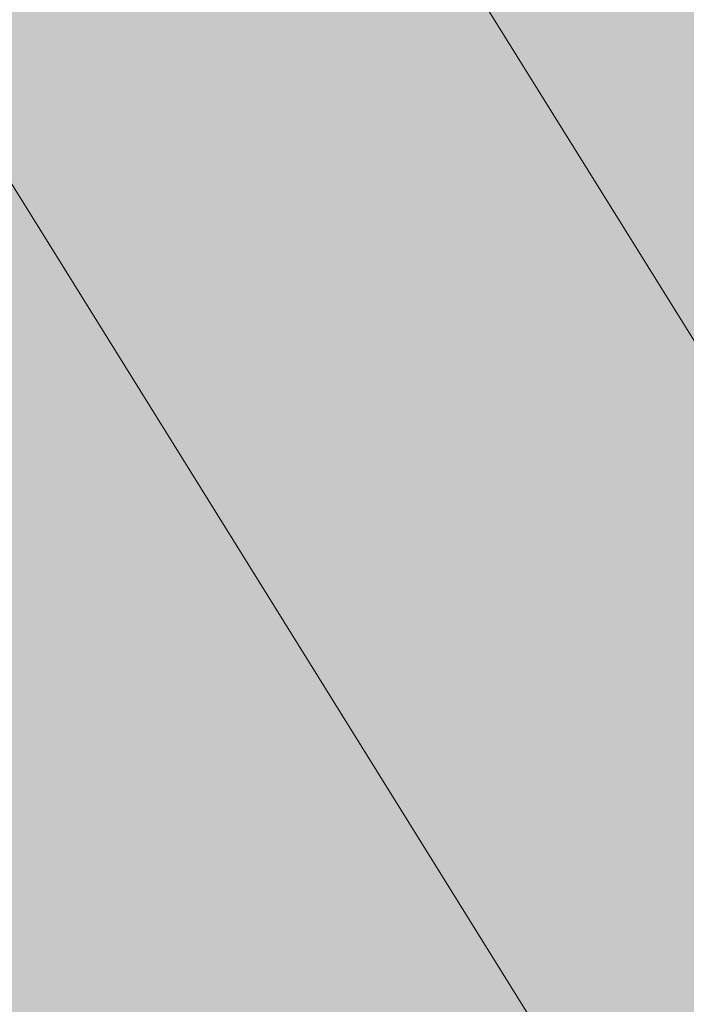
# Model space of a CAD drawing. Units: millimetres. Extents: x 11032 to 26788, y 3406 to 24505.
# Tile 49 of 78: x 15719 to 15786, y 16177 to 16276. Entities that reach past the tile are written whole.
import ezdxf

# ---------------------------------------------------------------- set-up
doc = ezdxf.new("R2010")
doc.units = ezdxf.units.MM
doc.header["$MEASUREMENT"] = 0
for name, color, linetype, lineweight in [('A-ANNO-DIMS', 2, 'Continuous', 18), ('A-GLAZ', 250, 'Continuous', 20), ('A-ROOF', 7, 'Continuous', 30), ('A-WALL', 7, 'Continuous', 35), ('E-LITE', 7, 'Continuous', 18), ('E-LITE-PATT', 7, 'Continuous', 13)]:
    doc.layers.add(name, color=color, linetype=linetype, lineweight=lineweight)
doc.layers.add('A-GLAZ-FRAM-PATT', color=250, linetype='Continuous', lineweight=13, true_color=0x262627)
doc.layers.add('A-ROOF-PATT', color=9, linetype='Continuous', lineweight=13, true_color=0xc7c8ca)
doc.styles.get("Standard").update_dxf_attribs({"font": 'arial.ttf'})
doc.dimstyles.get("Standard").update_dxf_attribs({"dimtxt": 150, "dimasz": 100, "dimexe": 10, "dimexo": 5, "dimgap": 5, "dimtad": 0, "dimtih": 1, "dimtoh": 1, "dimdec": 0, "dimzin": 0, "dimdsep": 46, "dimtxsty": 'Standard', "dimcen": 0.09, "dimadec": 0, "dimazin": 0, "dimtfac": 1, "dimtdec": 0, "dimtofl": 0, "dimtmove": 0, "dimatfit": 3, "dimfxl": 1, "dimtolj": 1, "dimtzin": 0, "dimarcsym": 0})

# ---------------------------------------------------------------- blocks, each defined once
blk = doc.blocks.new('*D36')
at = {"layer": 'A-ANNO-DIMS', "color": 0, "lineweight": -2, "transparency": 16777216}
for p, q in [((12301.265, 17115.885), (12301.265, 24416.858)), ((25397.404, 4466.399), (25397.404, 24416.858)), ((12401.265, 24406.858), (18569.198, 24406.858)), ((25297.404, 24406.858), (19129.471, 24406.858))]:
    blk.add_line(p, q, dxfattribs=at)
at = {"layer": 'A-ANNO-DIMS', "color": 0, "transparency": 16777216}
for points in [[(12401.265, 24423.525), (12401.265, 24390.191), (12301.265, 24406.858)], [(25297.404, 24423.525), (25297.404, 24390.191), (25397.404, 24406.858)]]:
    blk.add_solid(points, dxfattribs=at)
at = {"layer": 'Defpoints', "color": 0, "transparency": 16777216}
for p in [(25397.404, 24406.858), (12301.265, 17110.885), (25397.404, 4461.399)]:
    blk.add_point(p, dxfattribs=at)
at = {"layer": 'A-ANNO-DIMS', "color": 0, "transparency": 16777216, "insert": (18849.334, 24406.858), "char_height": 150, "attachment_point": 5}
blk.add_mtext('\\A1;13096', dxfattribs=at)
blk = doc.blocks.new('*D37')
at = {"layer": 'A-ANNO-DIMS', "color": 0, "lineweight": -2, "transparency": 16777216}
for p, q in [((18087.739, 23450.358), (11334.765, 23450.358)), ((11344.765, 23350.358), (11344.765, 14037.465)), ((11344.765, 4561.399), (11344.765, 13874.293)), ((12927.665, 4461.399), (11334.765, 4461.399))]:
    blk.add_line(p, q, dxfattribs=at)
at = {"layer": 'A-ANNO-DIMS', "color": 0, "transparency": 16777216}
for points in [[(11328.098, 23350.358), (11361.431, 23350.358), (11344.765, 23450.358)], [(11328.098, 4561.399), (11361.431, 4561.399), (11344.765, 4461.399)]]:
    blk.add_solid(points, dxfattribs=at)
at = {"layer": 'Defpoints', "color": 0, "transparency": 16777216}
for p in [(11344.765, 23450.358), (18092.739, 23450.358), (12932.665, 4461.399)]:
    blk.add_point(p, dxfattribs=at)
at = {"layer": 'A-ANNO-DIMS', "color": 0, "transparency": 16777216, "insert": (11344.765, 13955.879), "char_height": 150, "attachment_point": 5}
blk.add_mtext('\\A1;18989', dxfattribs=at)
blk = doc.blocks.new('*D45')
at = {"layer": 'A-ANNO-DIMS', "color": 0, "lineweight": -2, "transparency": 16777216}
for p, q in [((13792.367, 18518.925), (26363.904, 18518.925)), ((26353.904, 18418.925), (26353.904, 17450.319)), ((26353.904, 16318.44), (26353.904, 17287.045)), ((22902.404, 16218.44), (26363.904, 16218.44))]:
    blk.add_line(p, q, dxfattribs=at)
at = {"layer": 'A-ANNO-DIMS', "color": 0, "transparency": 16777216}
for points in [[(26337.237, 18418.925), (26370.57, 18418.925), (26353.904, 18518.925)], [(26337.237, 16318.44), (26370.57, 16318.44), (26353.904, 16218.44)]]:
    blk.add_solid(points, dxfattribs=at)
at = {"layer": 'Defpoints', "color": 0, "transparency": 16777216}
for p in [(13787.367, 18518.925), (26353.904, 18518.925), (22897.404, 16218.44)]:
    blk.add_point(p, dxfattribs=at)
at = {"layer": 'A-ANNO-DIMS', "color": 0, "transparency": 16777216, "insert": (26353.904, 17368.682), "char_height": 150, "attachment_point": 5}
blk.add_mtext('\\A1;2300.5', dxfattribs=at)
blk = doc.blocks.new('*D57')
at = {"layer": 'A-ANNO-DIMS', "color": 0, "lineweight": -2, "transparency": 16777216}
for p, q in [((14994.704, 7266.399), (14994.704, 24416.858)), ((20894.704, 7266.399), (20894.704, 24416.858)), ((15094.704, 24406.858), (17715.983, 24406.858)), ((20794.704, 24406.858), (18173.425, 24406.858))]:
    blk.add_line(p, q, dxfattribs=at)
at = {"layer": 'A-ANNO-DIMS', "color": 0, "transparency": 16777216}
for points in [[(15094.704, 24423.525), (15094.704, 24390.191), (14994.704, 24406.858)], [(20794.704, 24423.525), (20794.704, 24390.191), (20894.704, 24406.858)]]:
    blk.add_solid(points, dxfattribs=at)
at = {"layer": 'Defpoints', "color": 0, "transparency": 16777216}
for p in [(20894.704, 24406.858), (14994.704, 7261.399), (20894.704, 7261.399)]:
    blk.add_point(p, dxfattribs=at)
at = {"layer": 'A-ANNO-DIMS', "color": 0, "transparency": 16777216, "insert": (17944.704, 24406.858), "char_height": 150, "attachment_point": 5}
blk.add_mtext('\\A1;5900', dxfattribs=at)
blk = doc.blocks.new('*D60')
at = {"layer": 'A-ANNO-DIMS', "color": 0, "lineweight": -2, "transparency": 16777216}
for p, q in [((14994.704, 7266.399), (14994.704, 24416.858)), ((16344.704, 7266.399), (16344.704, 24416.858)), ((15094.704, 24406.858), (15448.043, 24406.858)), ((16244.704, 24406.858), (15891.365, 24406.858))]:
    blk.add_line(p, q, dxfattribs=at)
at = {"layer": 'A-ANNO-DIMS', "color": 0, "transparency": 16777216}
for points in [[(15094.704, 24423.525), (15094.704, 24390.191), (14994.704, 24406.858)], [(16244.704, 24423.525), (16244.704, 24390.191), (16344.704, 24406.858)]]:
    blk.add_solid(points, dxfattribs=at)
at = {"layer": 'Defpoints', "color": 0, "transparency": 16777216}
for p in [(16344.704, 24406.858), (14994.704, 7261.399), (16344.704, 7261.399)]:
    blk.add_point(p, dxfattribs=at)
at = {"layer": 'A-ANNO-DIMS', "color": 0, "transparency": 16777216, "insert": (15669.704, 24406.858), "char_height": 150, "attachment_point": 5}
blk.add_mtext('\\A1;1350', dxfattribs=at)

msp = doc.modelspace()

# ---------------------------------------------------------------- hatches: boundary and pattern name
at = {"layer": 'A-GLAZ-FRAM-PATT'}
h = msp.add_hatch(color=256, dxfattribs=at)
edge = h.paths.add_edge_path()
edge.add_line((15284.393, 17051.32), (15084.393, 17001.32))
edge.add_line((15084.393, 17001.32), (15084.393, 15951.32))
edge.add_spline(control_points=[(15084.393, 15951.32), (15157.266, 15924.219), (15224.458, 15897.808), (15284.393, 15870.289)], knot_values=[511.94901, 511.94901, 511.94901, 511.94901, 697.371598, 697.371598, 697.371598, 697.371598], degree=3, periodic=0)
edge.add_line((15284.393, 15870.289), (15284.393, 17051.32))
edge = h.paths.add_edge_path()
edge.add_line((15659.393, 16354.387), (15459.393, 16675.629))
edge.add_line((15459.393, 16675.629), (15459.393, 15771.505))
edge.add_spline(control_points=[(15459.393, 15771.505), (15501.891, 15741.568), (15571.096, 15682.692), (15632.72, 15612.509), (15659.393, 15578.299)], knot_values=[905.064582, 905.064582, 905.064582, 905.064582, 1079.468271, 1223.158435, 1223.158435, 1223.158435, 1223.158435], degree=3, periodic=0)
edge.add_line((15659.393, 15578.299), (15659.393, 16354.387))
h.paths.add_polyline_path([(15284.393, 17051.32), (15284.393, 16956.717), (15784.393, 16153.61), (15784.393, 16248.213)])
h = msp.add_hatch(color=256, dxfattribs=at)
edge = h.paths.add_edge_path()
edge.add_spline(control_points=[(15409.393, 16728.446), (15384.197, 16718.122), (15359.177, 16707.259), (15334.393, 16695.842)], knot_values=[2052.671403, 2052.671403, 2052.671403, 2052.671403, 2131.020164, 2131.020164, 2131.020164, 2131.020164], degree=3, periodic=0)
edge.add_line((15334.393, 16695.842), (15334.393, 15846.165))
edge.add_spline(control_points=[(15334.393, 15846.165), (15360.99, 15832.635), (15385.89, 15818.741), (15409.393, 15804.345)], knot_values=[750.83835, 750.83835, 750.83835, 750.83835, 839.475874, 839.475874, 839.475874, 839.475874], degree=3, periodic=0)
edge.add_line((15409.393, 15804.345), (15409.393, 16728.446))
edge = h.paths.add_edge_path()
edge.add_line((15784.393, 16153.61), (15709.393, 16274.076))
edge.add_line((15709.393, 16274.076), (15709.393, 15509.31))
edge.add_spline(control_points=[(15709.393, 15509.31), (15712.398, 15504.862), (15738.373, 15465.922), (15763.422, 15424.165), (15784.393, 15385.996)], knot_values=[1315.342429, 1315.342429, 1315.342429, 1315.342429, 1332.382415, 1463.285048, 1463.285048, 1463.285048, 1463.285048], degree=3, periodic=0)
edge.add_line((15784.393, 15385.996), (15784.393, 16153.61))
h = msp.add_hatch(color=256, dxfattribs=at)
edge = h.paths.add_edge_path()
edge.add_line((15784.393, 16248.213), (15784.393, 16153.61))
edge.add_line((15784.393, 16153.61), (16560.042, 14907.752))
edge.add_spline(control_points=[(16560.042, 14907.752), (16569.192, 14907.664), (16578.343, 14907.575), (16587.493, 14907.486), (16598.103, 14907.383), (16608.713, 14907.281), (16619.296, 14907.181)], knot_values=[1012.287873, 1012.287873, 1012.287873, 1012.287873, 1027.155312, 1027.155312, 1027.155312, 1044.393945, 1044.393945, 1044.393945, 1044.393945], degree=3, periodic=0)
edge.add_line((16619.296, 14907.181), (15784.393, 16248.213))
at = {"layer": 'A-ROOF-PATT'}
h = msp.add_hatch(color=256, dxfattribs=at)
edge = h.paths.add_edge_path()
edge.add_spline(control_points=[(17532.827, 17324.837), (17391.335, 17349.016), (16840.872, 17494.912), (16080.055, 18069.544), (14738.803, 18299.641), (13382.429, 18838.336), (12580.532, 17870.207), (12430.422, 17563.822)], knot_values=[2977.602794, 2977.602794, 2977.602794, 2977.602794, 3438.18406, 4811.646302, 5622.867548, 7588.028819, 8560.668579, 8560.668579, 8560.668579, 8560.668579], degree=3, periodic=0)
edge.add_spline(control_points=[(12430.422, 17563.822), (12437.904, 17573.36), (12445.386, 17582.899), (12452.869, 17592.437), (12452.869, 17592.438), (12452.869, 17592.438), (12452.869, 17592.438)], knot_values=[1408.564138, 1408.564138, 1408.564138, 1408.564138, 1444.85989, 1444.85989, 1444.85989, 1444.860118, 1444.860118, 1444.860118, 1444.860118], degree=3, periodic=0)
edge.add_spline(control_points=[(12452.869, 17592.438), (12555.432, 17723.185), (12736.557, 17929.686), (13044.86, 18114.643), (13219.943, 18189.644), (13299.92, 18220.646)], knot_values=[339.318246, 339.318246, 339.318246, 339.318246, 836.834997, 1151.251293, 1408.564138, 1408.564138, 1408.564138, 1408.564138], degree=3, periodic=0)
edge.add_spline(control_points=[(13299.92, 18220.646), (13299.998, 18220.689), (13300.077, 18220.732), (13319.738, 18231.488), (13339.24, 18241.402), (13388.645, 18264.703), (13418.466, 18277.069), (13478.019, 18298.648), (13507.751, 18307.861), (13544.561, 18317.488), (13551.584, 18319.245), (13558.612, 18320.924)], knot_values=[3783.895097, 3783.895097, 3783.895097, 3783.895097, 3784.17371, 3784.17371, 3853.466675, 3853.466675, 3960.240192, 3960.240192, 4067.013709, 4067.013709, 4092.174465, 4092.174465, 4092.174465, 4092.174465], degree=3, periodic=0)
edge.add_spline(control_points=[(13558.612, 18320.924), (13581.407, 18326.373), (13604.25, 18331.007), (13657.184, 18339.957), (13687.338, 18343.732), (13748.098, 18348.892), (13778.704, 18350.276), (13840.46, 18350.833), (13871.609, 18350.005), (13934.496, 18346.313), (13966.232, 18343.449), (14030.297, 18335.871), (14062.625, 18331.158), (14127.853, 18320.088), (14160.753, 18313.73), (14241.357, 18296.556), (14289.343, 18284.997), (14386.31, 18259.688), (14435.291, 18245.941), (14534.161, 18217.034), (14584.049, 18201.875), (14684.682, 18170.964), (14735.427, 18155.212), (14837.763, 18123.971), (14889.354, 18108.482), (14954.971, 18089.677), (14968.586, 18085.823), (14992.391, 18079.184), (15002.566, 18076.376), (15021.739, 18071.153), (15030.731, 18068.729), (15047.707, 18064.21), (15055.694, 18062.106), (15079.815, 18055.825), (15095.905, 18051.728), (15143.966, 18039.717), (15175.729, 18032.084), (15254.84, 18013.501), (15301.798, 18002.866), (15394.186, 17981.845), (15439.615, 17971.459), (15528.833, 17950.135), (15572.62, 17939.197), (15658.477, 17916.021), (15700.546, 17903.785), (15753.633, 17886.734), (15765.446, 17882.835), (15786.574, 17875.653), (15795.915, 17872.404), (15810.108, 17867.349), (15814.99, 17865.588), (15824.736, 17862.029), (15829.611, 17860.226), (15844.241, 17854.75), (15854.002, 17851.008), (15883.312, 17839.521), (15902.885, 17831.512), (15966.355, 17804.548), (16010.39, 17784.302), (16098.838, 17741.267), (16143.25, 17718.478), (16232.497, 17671.098), (16277.332, 17646.507), (16367.515, 17596.295), (16412.862, 17570.676), (16504.202, 17519.209), (16550.194, 17493.362), (16643.009, 17442.263), (16689.831, 17417.011), (16756.517, 17382.472), (16775.937, 17372.58), (16795.455, 17362.84)], knot_values=[4092.174465, 4092.174465, 4092.174465, 4092.174465, 4173.787226, 4173.787226, 4280.560743, 4280.560743, 4387.33426, 4387.33426, 4494.107777, 4494.107777, 4600.881294, 4600.881294, 4707.654811, 4707.654811, 4814.428328, 4814.428328, 4967.12624, 4967.12624, 5119.824153, 5119.824153, 5272.522066, 5272.522066, 5425.219978, 5425.219978, 5577.917891, 5577.917891, 5617.785332, 5617.785332, 5647.464848, 5647.464848, 5673.611025, 5673.611025, 5696.747607, 5696.747607, 5743.68189, 5743.68189, 5837.550457, 5837.550457, 5979.726105, 5979.726105, 6121.901752, 6121.901752, 6264.0774, 6264.0774, 6406.253047, 6406.253047, 6447.258585, 6447.258585, 6480.042088, 6480.042088, 6497.307706, 6497.307706, 6514.573324, 6514.573324, 6549.10456, 6549.10456, 6618.167032, 6618.167032, 6772.661017, 6772.661017, 6927.155002, 6927.155002, 7081.648987, 7081.648987, 7236.142972, 7236.142972, 7390.636957, 7390.636957, 7545.130942, 7545.130942, 7608.199287, 7608.199287, 7608.199287, 7608.199287], degree=3, periodic=0)
edge.add_spline(control_points=[(16795.455, 17362.84), (16814.335, 17349.456), (16832.897, 17336.263), (16873.225, 17307.197), (16894.778, 17291.386), (16936.221, 17259.941), (16956.11, 17244.308), (16993.863, 17213.094), (17011.726, 17197.514), (17041.993, 17169.265), (17054.791, 17156.601), (17078.762, 17131.225), (17089.933, 17118.516), (17110.618, 17092.991), (17120.131, 17080.178), (17130.17, 17065.264), (17131.487, 17063.277), (17133.77, 17059.776), (17134.746, 17058.261), (17136.69, 17055.205), (17137.657, 17053.668), (17140.539, 17049.025), (17142.438, 17045.89), (17148.068, 17036.367), (17151.732, 17029.859), (17163.03, 17008.788), (17170.335, 16993.646), (17184.087, 16961.978), (17190.534, 16945.453), (17202.562, 16911.165), (17208.142, 16893.402), (17218.448, 16856.821), (17223.173, 16838.003), (17231.801, 16799.51), (17235.705, 16779.837), (17241.533, 16746.739), (17243.676, 16733.5), (17247.718, 16706.37), (17249.608, 16692.472), (17252.066, 16672.69), (17252.761, 16666.875), (17254.1, 16655.226), (17254.744, 16649.4), (17256.596, 16631.917), (17257.727, 16620.254), (17260.823, 16585.238), (17262.489, 16561.858), (17266.551, 16488.654), (17267.658, 16438.661), (17267.349, 16375.228), (17267.193, 16362.07), (17266.95, 16348.891)], knot_values=[15.113047, 15.113047, 15.113047, 15.113047, 82.699515, 82.699515, 165.399029, 165.399029, 248.098544, 248.098544, 330.798058, 330.798058, 397.941946, 397.941946, 465.085833, 465.085833, 532.229721, 532.229721, 542.533741, 542.533741, 550.356816, 550.356816, 558.179891, 558.179891, 573.82604, 573.82604, 605.118339, 605.118339, 672.764061, 672.764061, 740.409783, 740.409783, 808.055505, 808.055505, 875.701227, 875.701227, 943.346949, 943.346949, 987.661349, 987.661349, 1033.412161, 1033.412161, 1052.385088, 1052.385088, 1071.358014, 1071.358014, 1109.303867, 1109.303867, 1185.195572, 1185.195572, 1346.441903, 1346.441903, 1388.558663, 1388.558663, 1388.558663, 1388.558663], degree=3, periodic=0)
edge.add_spline(control_points=[(17266.95, 16348.891), (17266.95, 16348.891), (17266.95, 16348.891), (17266.95, 16348.891), (17253.182, 15602.417), (17239.414, 14855.943), (17225.646, 14109.469)], knot_values=[1388.558663, 1388.558663, 1388.558663, 1388.558663, 1388.558965, 1388.558965, 1388.558965, 3774.076766, 3774.076766, 3774.076766, 3774.076766], degree=3, periodic=0)
edge.add_spline(control_points=[(17225.646, 14109.469), (17226.198, 14109.827), (17226.748, 14110.185), (17242.065, 14120.191), (17255.956, 14130.116), (17274.422, 14144.286), (17279.609, 14148.386), (17284.686, 14152.511)], knot_values=[1926.342397, 1926.342397, 1926.342397, 1926.342397, 1927.316729, 1927.316729, 1953.512176, 1953.512176, 1964.073235, 1964.073235, 1964.073235, 1964.073235], degree=3, periodic=0)
edge.add_spline(control_points=[(17284.686, 14152.511), (17315.791, 14194.761), (17384.413, 14446.273), (17407.128, 14793.401), (17407.093, 15295.84), (17423.274, 15626.362), (17415.601, 15782.507)], knot_values=[0, 0, 0, 0, 163.255467, 619.229677, 1171.862448, 1621.635556, 1621.635556, 1621.635556, 1621.635556], degree=3, periodic=0)
edge.add_spline(control_points=[(17415.601, 15782.507), (17438.21, 16077.57), (17410.495, 16533.484), (17390.893, 17030.649), (17301.082, 17169.349)], knot_values=[543.978475, 543.978475, 543.978475, 543.978475, 1452.985277, 1960.011493, 1960.011493, 1960.011493, 1960.011493], degree=3, periodic=0)
edge.add_spline(control_points=[(17301.082, 17169.349), (17346.58, 17157.64), (17392.235, 17147.336), (17467.161, 17132.609), (17496.336, 17127.412), (17525.58, 17122.709)], knot_values=[8131.593939, 8131.593939, 8131.593939, 8131.593939, 8269.734927, 8269.734927, 8357.501665, 8357.501665, 8357.501665, 8357.501665], degree=3, periodic=0)
edge.add_line((17525.58, 17122.709), (17532.827, 17324.837))
edge = h.paths.add_edge_path(flags=17)
edge.add_spline(control_points=[(13340.537, 14602.706), (13316.172, 14726.456), (13323.666, 14932.342), (13637.836, 15081.117), (13863.248, 15171.051), (14002.1, 15224.503), (14058.539, 15244.876)], knot_values=[680.893186, 680.893186, 680.893186, 680.893186, 1033.472829, 1337.400833, 1604.721426, 1784.294472, 1784.294472, 1784.294472, 1784.294472], degree=3, periodic=0)
edge.add_spline(control_points=[(14058.539, 15244.876), (14058.289, 15275.236), (14057.634, 15305.434), (14055.312, 15376.527), (14053.359, 15417.248), (14048.642, 15497.048), (14045.89, 15536.143), (14042.888, 15574.619)], knot_values=[6573.106542, 6573.106542, 6573.106542, 6573.106542, 6636.733001, 6636.733001, 6723.889055, 6723.889055, 6809.632877, 6809.632877, 6809.632877, 6809.632877], degree=3, periodic=0)
edge.add_spline(control_points=[(14042.888, 15574.619), (13546.54, 15403.221), (13074.735, 15143.241), (13277.36, 14695.339), (13340.537, 14602.706)], knot_values=[503.792578, 503.792578, 503.792578, 503.792578, 1728.178761, 2051.34844, 2051.34844, 2051.34844, 2051.34844], degree=3, periodic=0)
h = msp.add_hatch(color=256, dxfattribs=at)
h.set_gradient(color1=(254, 234, 185), color2=(254, 204, 102), name='HEMISPHERICAL')
edge = h.paths.add_edge_path()
edge.add_line((15084.393, 17001.32), (15284.393, 17051.32))
edge.add_line((15284.393, 17051.32), (15470.537, 16752.334))
edge.add_spline(control_points=[(15470.537, 16752.334), (15683.311, 16831.508), (16106.827, 16912.335), (16625.609, 16876.997), (17083.498, 16357.78), (17257.801, 16180.113)], knot_values=[0, 0, 0, 0, 655.293633, 1252.015784, 1989.616286, 1989.616286, 1989.616286, 1989.616286], degree=3, periodic=0)
edge.add_spline(control_points=[(17257.801, 16180.113), (17260.851, 16236.372), (17263.9, 16292.632), (17266.95, 16348.891)], knot_values=[1132.996772, 1132.996772, 1132.996772, 1132.996772, 1198.046422, 1198.046422, 1198.046422, 1198.046422], degree=3, periodic=0)
edge.add_spline(control_points=[(17266.95, 16348.891), (17267.193, 16362.07), (17267.349, 16375.228), (17267.658, 16438.661), (17266.551, 16488.654), (17262.489, 16561.858), (17260.823, 16585.238), (17257.727, 16620.254), (17256.596, 16631.917), (17254.744, 16649.4), (17254.1, 16655.226), (17252.761, 16666.875), (17252.066, 16672.69), (17249.608, 16692.472), (17247.718, 16706.37), (17243.676, 16733.5), (17241.533, 16746.739), (17235.705, 16779.837), (17231.801, 16799.51), (17223.173, 16838.003), (17218.448, 16856.821), (17208.142, 16893.402), (17202.562, 16911.165), (17190.534, 16945.453), (17184.087, 16961.978), (17170.335, 16993.646), (17163.03, 17008.788), (17151.732, 17029.859), (17148.068, 17036.367), (17142.438, 17045.89), (17140.539, 17049.025), (17137.657, 17053.668), (17136.69, 17055.205), (17134.746, 17058.261), (17133.77, 17059.776), (17131.487, 17063.277), (17130.17, 17065.264), (17120.131, 17080.178), (17110.618, 17092.991), (17089.933, 17118.516), (17078.762, 17131.225), (17054.791, 17156.601), (17041.993, 17169.265), (17011.726, 17197.514), (16993.863, 17213.094), (16956.11, 17244.308), (16936.221, 17259.941), (16894.778, 17291.386), (16873.225, 17307.197), (16832.897, 17336.263), (16814.335, 17349.456), (16795.455, 17362.84)], knot_values=[15.113047, 15.113047, 15.113047, 15.113047, 57.229808, 57.229808, 218.476138, 218.476138, 294.367844, 294.367844, 332.313696, 332.313696, 351.286623, 351.286623, 370.259549, 370.259549, 416.010361, 416.010361, 460.324761, 460.324761, 527.970483, 527.970483, 595.616205, 595.616205, 663.261927, 663.261927, 730.907649, 730.907649, 798.553371, 798.553371, 829.84567, 829.84567, 845.49182, 845.49182, 853.314895, 853.314895, 861.137969, 861.137969, 871.441989, 871.441989, 938.585877, 938.585877, 1005.729765, 1005.729765, 1072.873652, 1072.873652, 1155.573167, 1155.573167, 1238.272681, 1238.272681, 1320.972196, 1320.972196, 1388.558663, 1388.558663, 1388.558663, 1388.558663], degree=3, periodic=0)
edge.add_spline(control_points=[(16795.455, 17362.84), (16775.937, 17372.58), (16756.517, 17382.472), (16689.831, 17417.011), (16643.009, 17442.263), (16550.194, 17493.362), (16504.202, 17519.209), (16412.862, 17570.676), (16367.515, 17596.295), (16277.332, 17646.507), (16232.497, 17671.098), (16143.25, 17718.478), (16098.838, 17741.267), (16010.39, 17784.302), (15966.355, 17804.548), (15902.885, 17831.512), (15883.312, 17839.521), (15854.002, 17851.008), (15844.241, 17854.75), (15829.611, 17860.226), (15824.736, 17862.029), (15814.99, 17865.588), (15810.108, 17867.349), (15795.915, 17872.404), (15786.574, 17875.653), (15765.446, 17882.835), (15753.633, 17886.734), (15700.546, 17903.785), (15658.477, 17916.021), (15572.62, 17939.197), (15528.833, 17950.135), (15439.615, 17971.459), (15394.186, 17981.845), (15301.798, 18002.866), (15254.84, 18013.501), (15175.729, 18032.084), (15143.966, 18039.717), (15095.905, 18051.728), (15079.815, 18055.825), (15055.694, 18062.106), (15047.707, 18064.21), (15030.731, 18068.729), (15021.739, 18071.153), (15002.566, 18076.376), (14992.391, 18079.184), (14968.586, 18085.823), (14954.971, 18089.677), (14889.354, 18108.482), (14837.763, 18123.971), (14735.427, 18155.212), (14684.682, 18170.964), (14584.049, 18201.875), (14534.161, 18217.034), (14435.291, 18245.941), (14386.31, 18259.688), (14289.343, 18284.997), (14241.357, 18296.556), (14160.753, 18313.73), (14127.853, 18320.088), (14062.625, 18331.158), (14030.297, 18335.871), (13966.232, 18343.449), (13934.496, 18346.313), (13871.609, 18350.005), (13840.46, 18350.833), (13778.704, 18350.276), (13748.098, 18348.892), (13687.338, 18343.732), (13657.184, 18339.957), (13604.25, 18331.007), (13581.407, 18326.373), (13558.612, 18320.924)], knot_values=[4092.174465, 4092.174465, 4092.174465, 4092.174465, 4155.24281, 4155.24281, 4309.736795, 4309.736795, 4464.23078, 4464.23078, 4618.724765, 4618.724765, 4773.21875, 4773.21875, 4927.712735, 4927.712735, 5082.20672, 5082.20672, 5151.269192, 5151.269192, 5185.800428, 5185.800428, 5203.066045, 5203.066045, 5220.331663, 5220.331663, 5253.115167, 5253.115167, 5294.120705, 5294.120705, 5436.296352, 5436.296352, 5578.472, 5578.472, 5720.647647, 5720.647647, 5862.823295, 5862.823295, 5956.691861, 5956.691861, 6003.626145, 6003.626145, 6026.762727, 6026.762727, 6052.908904, 6052.908904, 6082.58842, 6082.58842, 6122.455861, 6122.455861, 6275.153773, 6275.153773, 6427.851686, 6427.851686, 6580.549599, 6580.549599, 6733.247511, 6733.247511, 6885.945424, 6885.945424, 6992.718941, 6992.718941, 7099.492458, 7099.492458, 7206.265975, 7206.265975, 7313.039492, 7313.039492, 7419.813009, 7419.813009, 7526.586526, 7526.586526, 7608.199287, 7608.199287, 7608.199287, 7608.199287], degree=3, periodic=0)
edge.add_spline(control_points=[(13558.612, 18320.924), (13472.381, 18287.498), (13386.15, 18254.072), (13299.92, 18220.646), (13299.92, 18220.646), (13299.92, 18220.646), (13299.92, 18220.646)], knot_values=[61.883246, 61.883246, 61.883246, 61.883246, 339.317975, 339.317975, 339.317975, 339.318246, 339.318246, 339.318246, 339.318246], degree=3, periodic=0)
edge.add_spline(control_points=[(13299.92, 18220.646), (13219.943, 18189.644), (13044.86, 18114.643), (12736.557, 17929.686), (12555.432, 17723.185), (12452.869, 17592.438)], knot_values=[339.318246, 339.318246, 339.318246, 339.318246, 596.631091, 911.047387, 1408.564138, 1408.564138, 1408.564138, 1408.564138], degree=3, periodic=0)
edge.add_spline(control_points=[(12452.869, 17592.438), (12452.869, 17592.438), (12452.869, 17592.438), (12452.869, 17592.437), (12445.386, 17582.899), (12437.904, 17573.36), (12430.422, 17563.822)], knot_values=[1408.564138, 1408.564138, 1408.564138, 1408.564138, 1408.564366, 1408.564366, 1408.564366, 1444.860118, 1444.860118, 1444.860118, 1444.860118], degree=3, periodic=0)
edge.add_spline(control_points=[(12430.422, 17563.822), (12373.797, 17448.248), (12157.302, 16836.764), (12751.985, 16393.69), (13424.325, 15907.903), (14042.888, 15574.619)], knot_values=[0, 0, 0, 0, 366.899303, 1975.594108, 2977.602794, 2977.602794, 2977.602794, 2977.602794], degree=3, periodic=0)
edge.add_spline(control_points=[(14042.888, 15574.619), (14042.839, 15575.252), (14042.789, 15575.886), (14039.681, 15615.607), (14036.366, 15654.052), (14029.551, 15729.305), (14026.05, 15766.114), (14019.175, 15837.686), (14015.8, 15872.45), (13903.823, 16338.596)], knot_values=[6310.22615, 6310.22615, 6310.22615, 6310.22615, 6311.638381, 6311.638381, 6398.794435, 6398.794435, 6485.950488, 6485.950488, 6573.106542, 6573.106542, 6573.106542, 6573.106542], degree=3, periodic=0)
edge.add_spline(control_points=[(13903.823, 16338.596), (14237.315, 16236.889), (14456.623, 16167.555), (14614.196, 16115.84)], knot_values=[0, 0, 0, 0, 202.985342, 202.985342, 202.985342, 202.985342], degree=3, periodic=0)
edge.add_spline(control_points=[(14614.196, 16115.84), (14663.209, 16178.992), (14799.965, 16341.237), (14969.915, 16481.426), (15084.393, 16556.825)], knot_values=[2405.034504, 2405.034504, 2405.034504, 2405.034504, 2644.882697, 3039.270727, 3039.270727, 3039.270727, 3039.270727], degree=3, periodic=0)
edge.add_line((15084.393, 16556.825), (15084.393, 17001.32))
h.paths.add_polyline_path([(14195.599, 17606.181, -1), (14395.599, 17606.181, -1)], flags=16)
h.paths.add_polyline_path([(13310.178, 17032.97, -1), (13510.178, 17032.97, -1)], flags=16)
h = msp.add_hatch(color=256, dxfattribs=at)
h.set_gradient(color1=(254, 234, 185), color2=(254, 204, 102), name='HEMISPHERICAL')
edge = h.paths.add_edge_path()
edge.add_spline(control_points=[(16560.042, 14907.752), (16569.192, 14907.664), (16578.343, 14907.575), (16587.493, 14907.486), (16832.101, 14905.115), (17122.895, 14902.296), (16849.359, 14976.117), (16870.954, 15304.114), (17098.337, 15241.178), (17235.385, 15203.245)], knot_values=[0, 0, 0, 0, 14.867439, 14.867439, 14.867439, 412.294309, 487.334592, 708.6416, 1044.393945, 1044.393945, 1044.393945, 1044.393945], degree=3, periodic=0)
edge.add_line((16587.504, 14907.486), (16560.207, 14907.486))
edge.add_line((16560.207, 14907.486), (15784.393, 16153.61))
edge.add_line((15784.393, 16153.61), (15784.393, 15385.996))
edge.add_spline(control_points=[(15784.393, 15385.996), (15798.391, 15360.52), (15847.198, 15266.214), (15887.196, 15168.614), (15912.903, 15096.727)], knot_values=[1463.285048, 1463.285048, 1463.285048, 1463.285048, 1550.659771, 1779.959936, 1779.959936, 1779.959936, 1779.959936], degree=3, periodic=0)
edge.add_spline(control_points=[(15912.903, 15096.727), (15913.652, 15095.649), (15914.403, 15094.565), (15925.191, 15078.948), (15935.516, 15063.47), (15956.582, 15030.918), (15967.324, 15013.844), (15989.119, 14978.386), (16000.173, 14960.003), (16022.525, 14922.193), (16033.824, 14902.767), (16056.63, 14863.116), (16068.138, 14842.891), (16091.349, 14801.871), (16103.053, 14781.075), (16126.666, 14739.118), (16138.575, 14717.958), (16162.628, 14675.459), (16174.772, 14654.12), (16199.352, 14611.428), (16211.787, 14590.075), (16237.037, 14547.491), (16249.851, 14526.26), (16271.946, 14490.566), (16281.092, 14476.044), (16299.694, 14447.129), (16309.149, 14432.737), (16328.456, 14404.098), (16338.307, 14389.85), (16358.518, 14361.503), (16368.879, 14347.403), (16390.266, 14319.347), (16401.291, 14305.391), (16420.626, 14281.969), (16428.703, 14272.467), (16445.363, 14253.527), (16453.946, 14244.088), (16471.727, 14225.278), (16480.926, 14215.907), (16500.075, 14197.247), (16510.026, 14187.959), (16530.844, 14169.504), (16541.71, 14160.337), (16564.549, 14142.195), (16576.522, 14133.22), (16597.69, 14118.448), (16606.528, 14112.565), (16624.87, 14101.004), (16634.376, 14095.326), (16654.117, 14084.255), (16664.352, 14078.862), (16685.603, 14068.46), (16696.619, 14063.452), (16719.46, 14053.944), (16731.285, 14049.444), (16755.742, 14041.097), (16768.374, 14037.251), (16794.396, 14030.368), (16807.787, 14027.332), (16835.229, 14022.23), (16849.279, 14020.163), (16877.882, 14017.141), (16892.435, 14016.186), (16921.835, 14015.489), (16936.683, 14015.749), (16961.564, 14017.241), (16971.582, 14018.127), (16986.57, 14019.883), (16991.56, 14020.54), (16999.027, 14021.63), (17001.514, 14022.011), (17006.48, 14022.809), (17008.962, 14023.225), (17014.824, 14024.251), (17018.193, 14024.875), (17036.262, 14028.398), (17050.55, 14031.826), (17078.171, 14039.583), (17091.505, 14043.912), (17115.643, 14052.705), (17126.557, 14057.089), (17137.108, 14061.688)], knot_values=[2010.763962, 2010.763962, 2010.763962, 2010.763962, 2014.702983, 2014.702983, 2067.238337, 2067.238337, 2119.773691, 2119.773691, 2172.309046, 2172.309046, 2224.8444, 2224.8444, 2277.379754, 2277.379754, 2329.915109, 2329.915109, 2382.450463, 2382.450463, 2434.985817, 2434.985817, 2487.521172, 2487.521172, 2540.056526, 2540.056526, 2576.317929, 2576.317929, 2612.579332, 2612.579332, 2648.840735, 2648.840735, 2685.102138, 2685.102138, 2721.363541, 2721.363541, 2746.252015, 2746.252015, 2771.14049, 2771.14049, 2796.028964, 2796.028964, 2820.917439, 2820.917439, 2845.805913, 2845.805913, 2870.694388, 2870.694388, 2887.513276, 2887.513276, 2904.332164, 2904.332164, 2921.151052, 2921.151052, 2937.96994, 2937.96994, 2954.788828, 2954.788828, 2971.607717, 2971.607717, 2988.426605, 2988.426605, 3005.245493, 3005.245493, 3022.064381, 3022.064381, 3038.883269, 3038.883269, 3050.197545, 3050.197545, 3055.854683, 3055.854683, 3058.683252, 3058.683252, 3061.511821, 3061.511821, 3065.393417, 3065.393417, 3082.466872, 3082.466872, 3099.540326, 3099.540326, 3114.543344, 3114.543344, 3114.543344, 3114.543344], degree=3, periodic=0)
edge.add_spline(control_points=[(17137.108, 14061.688), (17165.253, 14274.398), (17209.97, 14653.885), (17230.2, 15035.586), (17235.385, 15203.245)], knot_values=[1968.080456, 1968.080456, 1968.080456, 1968.080456, 2611.528287, 3114.537926, 3114.537926, 3114.537926, 3114.537926], degree=3, periodic=0)
edge = h.paths.add_edge_path()
edge.add_spline(control_points=[(16856.103, 14956.992), (16852.841, 14961.219), (16849.83, 14965.576), (16842.539, 14977.287), (16838.658, 14984.798), (16832.033, 15000.109), (16829.289, 15007.911), (16824.126, 15026.008), (16822.047, 15036.354), (16819.308, 15057.097), (16818.649, 15067.496), (16818.576, 15088.188), (16819.162, 15098.483), (16821.467, 15118.823), (16823.186, 15128.868), (16827.696, 15148.567), (16830.486, 15158.22), (16836.065, 15173.969), (16838.565, 15180.211), (16844.079, 15192.402), (16847.092, 15198.353), (16852.029, 15207.021), (16853.744, 15209.868), (16857.321, 15215.468), (16859.188, 15218.226), (16863.017, 15223.558), (16864.978, 15226.136), (16872.565, 15235.558), (16878.593, 15241.952), (16891.428, 15253.591), (16898.232, 15258.834), (16912.397, 15268.127), (16919.756, 15272.176), (16934.816, 15279.138), (16942.515, 15282.052), (16958.1, 15286.873), (16965.985, 15288.78), (16984.013, 15292.142), (16994.186, 15293.334), (17014.631, 15294.619), (17024.904, 15294.713), (17048.453, 15293.935), (17061.76, 15292.783), (17088.519, 15289.422), (17101.972, 15287.211), (17131.961, 15281.46), (17148.526, 15277.734), (17181.692, 15269.627), (17198.292, 15265.245), (17222.182, 15258.759), (17229.535, 15256.737), (17236.862, 15254.714)], knot_values=[9.663953, 9.663953, 9.663953, 9.663953, 20.035167, 20.035167, 36.941175, 36.941175, 53.847184, 53.847184, 75.779569, 75.779569, 97.711954, 97.711954, 119.644339, 119.644339, 141.576724, 141.576724, 163.509109, 163.509109, 178.382995, 178.382995, 193.25688, 193.25688, 200.693823, 200.693823, 208.130766, 208.130766, 215.444859, 215.444859, 235.579592, 235.579592, 255.714326, 255.714326, 275.84906, 275.84906, 295.983794, 295.983794, 316.118527, 316.118527, 341.722054, 341.722054, 367.325581, 367.325581, 400.157243, 400.157243, 432.988905, 432.988905, 473.044017, 473.044017, 513.099128, 513.099128, 530.9693, 530.9693, 530.9693, 530.9693], degree=3, periodic=0)
edge.add_spline(control_points=[(17236.862, 15254.714), (17240.377, 15387.456), (17242.496, 15609.536), (17239.752, 15831.567), (17250.544, 16044.717)], knot_values=[1250.981862, 1250.981862, 1250.981862, 1250.981862, 1649.151658, 1916.613987, 1916.613987, 1916.613987, 1916.613987], degree=3, periodic=0)
edge.add_spline(control_points=[(17250.544, 16044.717), (17229.169, 16066.505), (17207.794, 16088.292), (17186.419, 16110.08), (17186.418, 16110.08), (17186.418, 16110.081), (17186.418, 16110.081)], knot_values=[-88.518558, -88.518558, -88.518558, -88.518558, -0.001278, -0.001278, -0.001278, 0, 0, 0, 0], degree=3, periodic=0)
edge.add_spline(control_points=[(17186.418, 16110.081), (17169.261, 16127.569), (17151.499, 16145.947), (17114.892, 16184.084), (17096.046, 16203.842), (17057.437, 16244.305), (17037.673, 16265.01), (16997.415, 16306.918), (16976.921, 16328.12), (16927.79, 16378.347), (16898.924, 16407.388), (16840.771, 16464.327), (16811.484, 16492.225), (16758.449, 16540.764), (16734.666, 16561.798), (16687.634, 16601.588), (16664.382, 16620.344), (16624.116, 16650.909), (16606.897, 16663.324), (16583.769, 16678.999), (16577.49, 16683.149), (16567.144, 16689.805), (16563.039, 16692.397), (16550.823, 16699.959), (16542.775, 16704.739), (16526.841, 16713.814), (16518.956, 16718.108), (16495.524, 16730.301), (16480.199, 16737.514), (16449.97, 16750.334), (16435.066, 16755.942), (16405.476, 16765.764), (16390.79, 16769.979), (16361.418, 16777.195), (16346.731, 16780.197), (16317.147, 16785.133), (16302.249, 16787.067), (16272.053, 16789.992), (16256.756, 16790.981), (16225.609, 16792.125), (16209.759, 16792.279), (16177.385, 16791.865), (16160.862, 16791.296), (16136.98, 16790.07), (16129.942, 16789.661), (16118.22, 16788.91), (16113.574, 16788.594), (16103.645, 16787.886), (16098.362, 16787.489), (16087.761, 16786.652), (16082.439, 16786.212), (16066.413, 16784.825), (16055.649, 16783.812), (16023.135, 16780.505), (16001.164, 16777.942), (15934.539, 16769.141), (15889.17, 16761.791), (15797.417, 16743.949), (15751.033, 16733.457), (15645.217, 16705.796), (15585.74, 16687.58), (15526.207, 16666.217), (15525.367, 16665.915), (15524.528, 16665.613)], knot_values=[0, 0, 0, 0, 71.050145, 71.050145, 142.100291, 142.100291, 213.150436, 213.150436, 284.200582, 284.200582, 381.323193, 381.323193, 478.445804, 478.445804, 557.821985, 557.821985, 637.198165, 637.198165, 698.312259, 698.312259, 721.397137, 721.397137, 736.779089, 736.779089, 767.542992, 767.542992, 798.306896, 798.306896, 859.834702, 859.834702, 921.362509, 921.362509, 982.890315, 982.890315, 1044.418122, 1044.418122, 1105.945928, 1105.945928, 1167.473735, 1167.473735, 1229.001542, 1229.001542, 1290.529348, 1290.529348, 1315.899004, 1315.899004, 1332.381279, 1332.381279, 1350.905266, 1350.905266, 1369.429252, 1369.429252, 1406.477225, 1406.477225, 1480.573171, 1480.573171, 1628.765063, 1628.765063, 1776.956955, 1776.956955, 1966.310925, 1966.310925, 1969.019495, 1969.019495, 1969.019495, 1969.019495], degree=3, periodic=0)
edge.add_line((15524.528, 16665.613), (16587.978, 14957.484))
edge.add_spline(control_points=[(16587.978, 14957.484), (16605.253, 14957.316), (16622.516, 14957.149), (16665.945, 14956.759), (16691.933, 14956.554), (16742.419, 14956.302), (16766.918, 14956.255), (16813.531, 14956.412), (16835.647, 14956.617), (16856.103, 14956.992)], knot_values=[872.218193, 872.218193, 872.218193, 872.218193, 900.28573, 900.28573, 943.365989, 943.365989, 986.446248, 986.446248, 1029.526506, 1029.526506, 1029.526506, 1029.526506], degree=3, periodic=0)
h.paths.add_polyline_path([(16474.605, 15622.642, -1), (16624.605, 15622.642, -1)], flags=16)
h.paths.add_polyline_path([(16198.536, 16037.613, -1), (16348.536, 16037.613, -1)], flags=16)
h.paths.add_polyline_path([(16475.717, 16408.125, -1), (16625.717, 16408.125, -1)], flags=16)
at = {"layer": 'E-LITE-PATT'}
h = msp.add_hatch(color=256, dxfattribs=at)
edge = h.paths.add_edge_path()
edge.add_spline(control_points=[(15084.393, 16556.825), (14969.915, 16481.426), (14799.965, 16341.237), (14663.209, 16178.992), (14614.196, 16115.84)], knot_values=[2405.034504, 2405.034504, 2405.034504, 2405.034504, 2799.422535, 3039.270727, 3039.270727, 3039.270727, 3039.270727], degree=3, periodic=0)
edge.add_spline(control_points=[(14614.196, 16115.84), (14650.957, 16103.776), (14684.357, 16092.67), (14715.064, 16082.336)], knot_values=[202.985342, 202.985342, 202.985342, 202.985342, 250.340862, 250.340862, 250.340862, 250.340862], degree=3, periodic=0)
edge.add_spline(control_points=[(14715.064, 16082.336), (14732.32, 16103.979), (14749.873, 16125.274), (14780.086, 16160.475), (14792.544, 16174.592), (14817.876, 16202.424), (14830.748, 16216.137), (14853.903, 16239.975), (14864.109, 16250.213), (14884.415, 16270.066), (14894.503, 16279.688), (14918.667, 16302.183), (14932.865, 16314.967), (14987.375, 16362.454), (15029.339, 16395.81), (15076.718, 16430.13), (15080.55, 16432.882), (15084.393, 16435.621)], knot_values=[2472.58551, 2472.58551, 2472.58551, 2472.58551, 2558.786533, 2558.786533, 2617.797515, 2617.797515, 2676.808498, 2676.808498, 2721.997624, 2721.997624, 2765.342439, 2765.342439, 2824.40593, 2824.40593, 2988.235172, 2988.235172, 3002.598788, 3002.598788, 3002.598788, 3002.598788], degree=3, periodic=0)
edge.add_line((15084.393, 16435.621), (15084.393, 16556.825))
edge = h.paths.add_edge_path()
edge.add_spline(control_points=[(17257.801, 16180.113), (17083.498, 16357.78), (16625.609, 16876.997), (16106.827, 16912.335), (15683.311, 16831.508), (15470.537, 16752.334)], knot_values=[0, 0, 0, 0, 737.600502, 1334.322652, 1989.616286, 1989.616286, 1989.616286, 1989.616286], degree=3, periodic=0)
edge.add_line((15470.537, 16752.334), (15524.528, 16665.613))
edge.add_spline(control_points=[(15524.528, 16665.613), (15525.367, 16665.915), (15526.207, 16666.217), (15585.74, 16687.58), (15645.217, 16705.796), (15751.033, 16733.457), (15797.417, 16743.949), (15889.17, 16761.791), (15934.539, 16769.141), (16001.164, 16777.942), (16023.135, 16780.505), (16055.649, 16783.812), (16066.413, 16784.825), (16082.439, 16786.212), (16087.761, 16786.652), (16098.362, 16787.489), (16103.645, 16787.886), (16113.574, 16788.594), (16118.22, 16788.91), (16129.942, 16789.661), (16136.98, 16790.07), (16160.862, 16791.296), (16177.385, 16791.865), (16209.759, 16792.279), (16225.609, 16792.125), (16256.756, 16790.981), (16272.053, 16789.992), (16302.249, 16787.067), (16317.147, 16785.133), (16346.731, 16780.197), (16361.418, 16777.195), (16390.79, 16769.979), (16405.476, 16765.764), (16435.066, 16755.942), (16449.97, 16750.334), (16480.199, 16737.514), (16495.524, 16730.301), (16518.956, 16718.108), (16526.841, 16713.814), (16542.775, 16704.739), (16550.823, 16699.959), (16563.039, 16692.397), (16567.144, 16689.805), (16577.49, 16683.149), (16583.769, 16678.999), (16606.897, 16663.324), (16624.116, 16650.909), (16664.382, 16620.344), (16687.634, 16601.588), (16734.666, 16561.798), (16758.449, 16540.764), (16811.484, 16492.225), (16840.771, 16464.327), (16898.924, 16407.388), (16927.79, 16378.347), (16976.921, 16328.12), (16997.415, 16306.918), (17037.673, 16265.01), (17057.437, 16244.305), (17096.046, 16203.842), (17114.892, 16184.084), (17151.499, 16145.947), (17169.261, 16127.569), (17186.418, 16110.081)], knot_values=[0, 0, 0, 0, 2.70857, 2.70857, 192.06254, 192.06254, 340.254432, 340.254432, 488.446324, 488.446324, 562.54227, 562.54227, 599.590243, 599.590243, 618.114229, 618.114229, 636.638216, 636.638216, 653.120491, 653.120491, 678.490147, 678.490147, 740.017953, 740.017953, 801.54576, 801.54576, 863.073567, 863.073567, 924.601373, 924.601373, 986.12918, 986.12918, 1047.656986, 1047.656986, 1109.184793, 1109.184793, 1170.712599, 1170.712599, 1201.476503, 1201.476503, 1232.240406, 1232.240406, 1247.622358, 1247.622358, 1270.707236, 1270.707236, 1331.82133, 1331.82133, 1411.19751, 1411.19751, 1490.573691, 1490.573691, 1587.696302, 1587.696302, 1684.818913, 1684.818913, 1755.869059, 1755.869059, 1826.919204, 1826.919204, 1897.96935, 1897.96935, 1969.019495, 1969.019495, 1969.019495, 1969.019495], degree=3, periodic=0)
edge.add_spline(control_points=[(17186.418, 16110.081), (17186.418, 16110.081), (17186.418, 16110.08), (17186.419, 16110.08), (17207.794, 16088.292), (17229.169, 16066.505), (17250.544, 16044.717)], knot_values=[-88.518558, -88.518558, -88.518558, -88.518558, -88.51728, -88.51728, -88.51728, 0, 0, 0, 0], degree=3, periodic=0)
edge.add_spline(control_points=[(17250.544, 16044.717), (17251.307, 16059.803), (17252.131, 16075.51), (17253.018, 16091.882)], knot_values=[1232.05171, 1232.05171, 1232.05171, 1232.05171, 1250.981862, 1250.981862, 1250.981862, 1250.981862], degree=3, periodic=0)
edge.add_spline(control_points=[(17253.018, 16091.882), (17253.019, 16091.892), (17253.019, 16091.901), (17253.02, 16091.911), (17254.614, 16121.312), (17256.207, 16150.712), (17257.801, 16180.113)], knot_values=[1198.046422, 1198.046422, 1198.046422, 1198.046422, 1198.057605, 1198.057605, 1198.057605, 1232.05171, 1232.05171, 1232.05171, 1232.05171], degree=3, periodic=0)

# ---------------------------------------------------------------- linework, layer by layer
at = {"layer": 'A-GLAZ'}
for p, q in [((15284.393, 17051.32), (16619.296, 14907.181)), ((15284.393, 16956.717), (16560.207, 14907.486))]:
    msp.add_line(p, q, dxfattribs=at)
at = {"layer": 'A-ROOF'}
msp.add_open_spline([(14042.888, 15574.619), (13424.325, 15907.903), (12751.985, 16393.69), (11963.048, 16981.495), (13249.687, 18891.056), (14738.803, 18299.641), (16080.055, 18069.544), (16966.203, 17400.251), (17654.208, 17293.942), (17944.704, 17286.735)], degree=3, knots=[0, 0, 0, 0, 1002.008686, 2610.703491, 3950.242555, 5915.403825, 6726.625071, 8100.087313, 8996.431878, 8996.431878, 8996.431878, 8996.431878], dxfattribs=at)
at = {"layer": 'A-WALL'}
msp.add_open_spline([(13903.823, 16338.596), (14592.588, 16128.54), (14947.845, 16001.782), (15353.854, 15853.294), (15563.925, 15701.294), (15714.647, 15512.154), (15830.664, 15306.558), (15887.196, 15168.614), (15912.903, 15096.727)], degree=3, knots=[0, 0, 0, 0, 419.227886, 738.351858, 1079.468271, 1332.382415, 1550.659771, 1779.959936, 1779.959936, 1779.959936, 1779.959936], dxfattribs=at)
at = {"layer": 'E-LITE'}
for points, knots in [([(17257.801, 16180.113), (17083.498, 16357.78), (16625.609, 16876.997), (16069.956, 16914.847), (15586.409, 16811.936), (15334.393, 16695.842)], [0, 0, 0, 0, 737.600502, 1334.322652, 2131.020164, 2131.020164, 2131.020164, 2131.020164]), ([(17250.544, 16044.717), (17229.169, 16066.505), (17207.794, 16088.292), (17186.419, 16110.08), (17186.418, 16110.08), (17186.418, 16110.081), (17186.418, 16110.081), (17169.261, 16127.569), (17151.499, 16145.947), (17114.892, 16184.084), (17096.046, 16203.842), (17057.437, 16244.305), (17037.673, 16265.01), (16997.415, 16306.918), (16976.921, 16328.12), (16927.79, 16378.347), (16898.924, 16407.388), (16840.771, 16464.327), (16811.484, 16492.225), (16758.449, 16540.764), (16734.666, 16561.798), (16687.634, 16601.588), (16664.382, 16620.344), (16624.116, 16650.909), (16606.897, 16663.324), (16583.769, 16678.999), (16577.49, 16683.149), (16567.144, 16689.805), (16563.039, 16692.397), (16550.823, 16699.959), (16542.775, 16704.739), (16526.841, 16713.814), (16518.956, 16718.108), (16495.524, 16730.301), (16480.199, 16737.514), (16449.97, 16750.334), (16435.066, 16755.942), (16405.476, 16765.764), (16390.79, 16769.979), (16361.418, 16777.195), (16346.731, 16780.197), (16317.147, 16785.133), (16302.249, 16787.067), (16272.053, 16789.992), (16256.756, 16790.981), (16225.609, 16792.125), (16209.759, 16792.279), (16177.385, 16791.865), (16160.862, 16791.296), (16136.98, 16790.07), (16129.942, 16789.661), (16118.22, 16788.91), (16113.574, 16788.594), (16103.645, 16787.886), (16098.362, 16787.489), (16087.761, 16786.652), (16082.439, 16786.212), (16066.413, 16784.825), (16055.649, 16783.812), (16023.135, 16780.505), (16001.164, 16777.942), (15934.539, 16769.141), (15889.17, 16761.791), (15797.417, 16743.949), (15751.033, 16733.457), (15645.217, 16705.796), (15585.74, 16687.58), (15526.207, 16666.217), (15525.367, 16665.915), (15524.528, 16665.613)], [-88.518558, -88.518558, -88.518558, -88.518558, -0.001278, -0.001278, -0.001278, 0, 0, 0, 71.050145, 71.050145, 142.100291, 142.100291, 213.150436, 213.150436, 284.200582, 284.200582, 381.323193, 381.323193, 478.445804, 478.445804, 557.821985, 557.821985, 637.198165, 637.198165, 698.312259, 698.312259, 721.397137, 721.397137, 736.779089, 736.779089, 767.542992, 767.542992, 798.306896, 798.306896, 859.834702, 859.834702, 921.362509, 921.362509, 982.890315, 982.890315, 1044.418122, 1044.418122, 1105.945928, 1105.945928, 1167.473735, 1167.473735, 1229.001542, 1229.001542, 1290.529348, 1290.529348, 1315.899004, 1315.899004, 1332.381279, 1332.381279, 1350.905266, 1350.905266, 1369.429252, 1369.429252, 1406.477225, 1406.477225, 1480.573171, 1480.573171, 1628.765063, 1628.765063, 1776.956955, 1776.956955, 1966.310925, 1966.310925, 1969.019495, 1969.019495, 1969.019495, 1969.019495])]:
    msp.add_open_spline(points, degree=3, knots=knots, dxfattribs=at)

# ---------------------------------------------------------------- dimensions: what is measured, and where the dimension line sits
at = {"layer": 'A-ANNO-DIMS'}
for base, p1, p2, picture, middle in [((25397.404, 24406.858), (12301.265, 17110.885), (25397.404, 4461.399), '*D36', (18849.334, 24406.858)), ((20894.704, 24406.858), (14994.704, 7261.399), (20894.704, 7261.399), '*D57', (17944.704, 24406.858)), ((16344.704, 24406.858), (14994.704, 7261.399), (16344.704, 7261.399), '*D60', (15669.704, 24406.858))]:
    dim = msp.add_linear_dim(base=base, p1=p1, p2=p2, dimstyle='Standard', override={"dimdec": 0, "dimlfac": 1, "dimrnd": 0, "dimzin": 0, "dimdsep": 46, "dimlunit": 2}, dxfattribs=at)
    dim.commit()
    dim.dimension.update_dxf_attribs({"geometry": picture, "text_midpoint": middle})
for base, p1, p2, override, picture, middle in [((11344.765, 23450.358), (12932.665, 4461.399), (18092.739, 23450.358), {"dimdec": 0, "dimlfac": 1, "dimrnd": 0, "dimzin": 0, "dimdsep": 46, "dimlunit": 2}, '*D37', (11344.765, 13955.879)), ((26353.904, 18518.925), (22897.404, 16218.44), (13787.367, 18518.925), {"dimdec": 1, "dimlfac": 1, "dimrnd": 0, "dimzin": 0, "dimdsep": 46, "dimlunit": 2}, '*D45', (26353.904, 17368.682))]:
    dim = msp.add_linear_dim(base=base, p1=p1, p2=p2, angle=90, dimstyle='Standard', override=override, dxfattribs=at)
    dim.commit()
    dim.dimension.update_dxf_attribs({"geometry": picture, "text_midpoint": middle})

doc.saveas('drawing.dxf')
